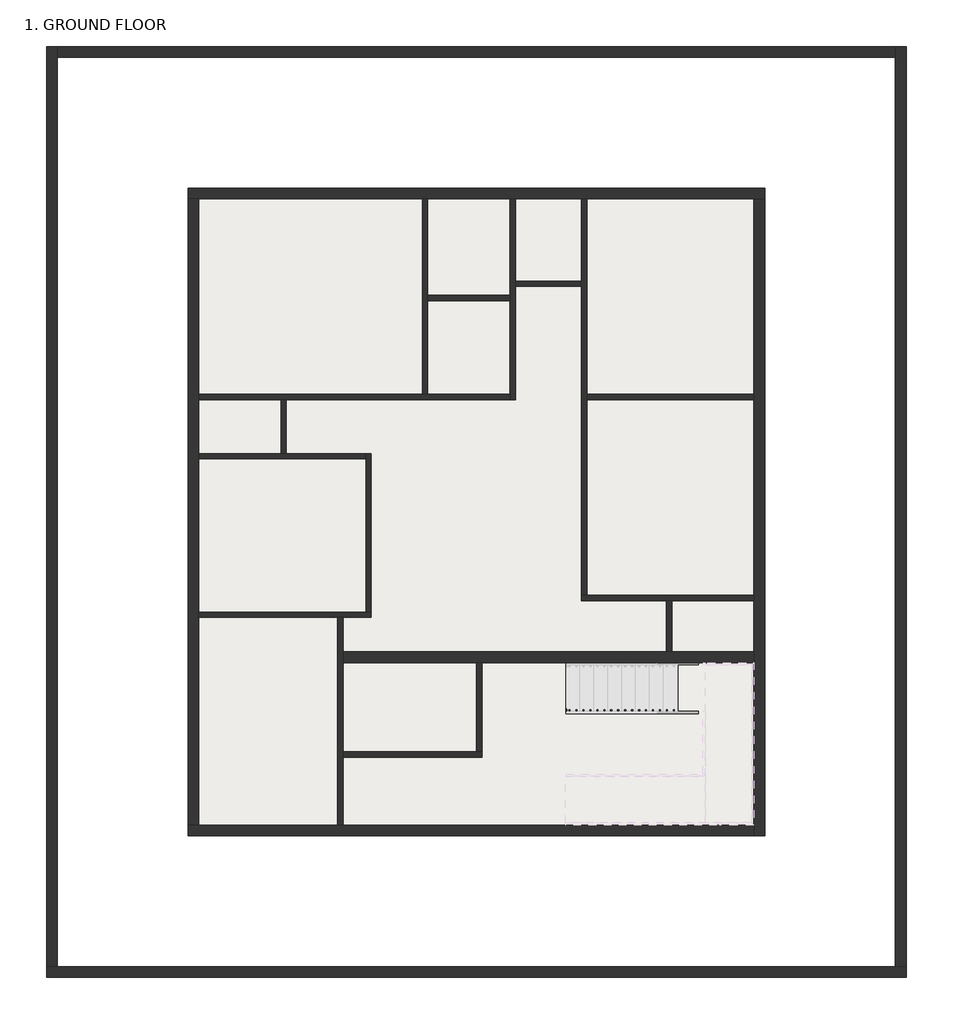
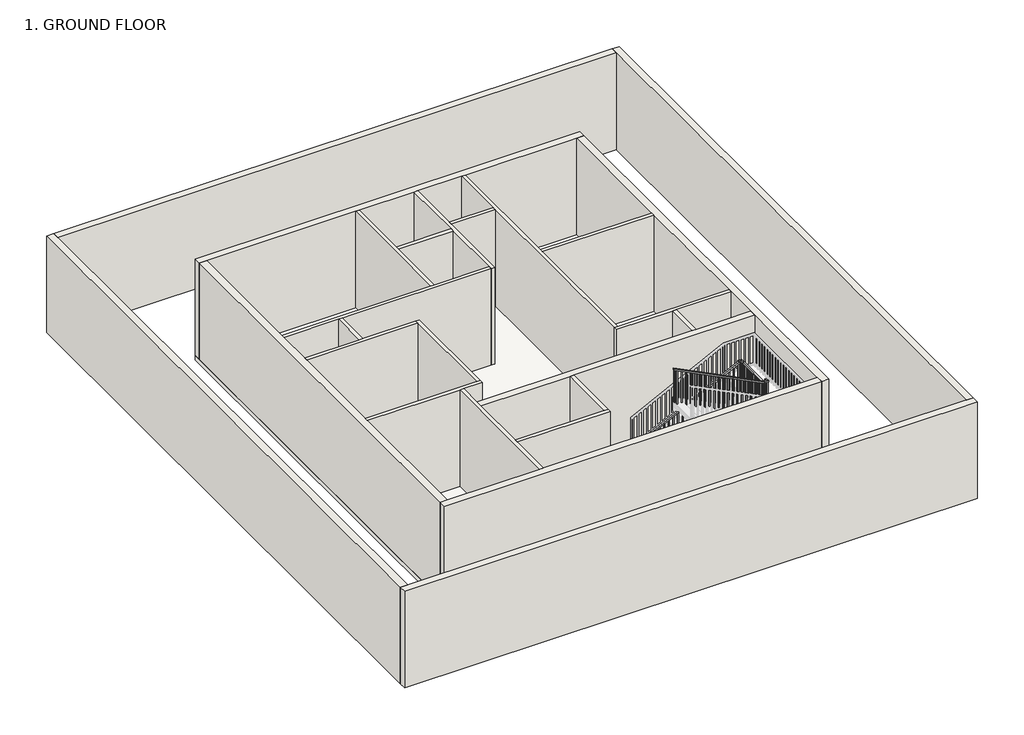
# One storey, part 1 of 2: 25 walls, 3 slabs, 1 railing.
"""IFC4 building model written with IfcOpenShell, lengths in millimetres."""

from ifc_helpers import new_model, si_unit, frame, origin, origin_with_axes, place, context, project, spatial, polyline, outline, extrude, faceted_brep, element, save

model = new_model("IFC4")

# Units and contexts
model_context = context("Model", 3, world=origin())
ifc_project = project(units=[si_unit("LENGTHUNIT", "METRE", prefix="MILLI")], contexts=[model_context])

# Site, building, storey
site = spatial("IfcSite", under=ifc_project)
building = spatial("IfcBuilding", under=site)
storey = spatial("IfcBuildingStorey", under=building, Name="1. GROUND FLOOR", Elevation=0.0)

# Railing
placement = place(None, origin())
element("IfcRailing", 1, ObjectType="1100mm", at=placement, inside=storey, context=model_context, shape_type="SolidModel", body=[
    faceted_brep([(1688.8435815, -3923.691395, 1250.0), (1688.8435815, -3923.691395, 1194.0983006), (1688.8435815, -3973.691395, 1194.0983006), (1688.8435815, -3973.691395, 1250.0), (4614.2435815, -3923.691395, 2712.7), (4664.2435815, -3923.691395, 2681.7983006), (4664.2435815, -3973.691395, 2681.7983006), (4614.2435815, -3973.691395, 2712.7), (4614.2435815, -3923.691395, 2750.0), (4664.2435815, -3923.691395, 2700.0), (4664.2435815, -3973.691395, 2700.0), (4614.2435815, -3973.691395, 2750.0), (4739.2435815, -3923.691395, 2750.0), (4739.2435815, -3923.691395, 2700.0), (4689.2435815, -3973.691395, 2700.0), (4689.2435815, -3973.691395, 2750.0), (4739.2435815, -4048.691395, 2750.0), (4739.2435815, -4048.691395, 2700.0), (4689.2435815, -4048.691395, 2700.0), (4689.2435815, -4048.691395, 2750.0), (4739.2435815, -5301.891395, 2750.0), (4739.2435815, -5351.891395, 2700.0), (4689.2435815, -5351.891395, 2700.0), (4689.2435815, -5301.891395, 2750.0), (4739.2435815, -5301.891395, 2937.3), (4739.2435815, -5351.891395, 2887.3), (4689.2435815, -5351.891395, 2887.3), (4689.2435815, -5301.891395, 2937.3), (4739.2435815, -5426.891395, 2937.3), (4739.2435815, -5426.891395, 2887.3), (4689.2435815, -5376.891395, 2887.3), (4689.2435815, -5376.891395, 2937.3), (4614.2435815, -5426.891395, 2937.3), (4602.4401826, -5426.891395, 2887.3), (4602.4401826, -5376.891395, 2887.3), (4614.2435815, -5376.891395, 2937.3), (1688.8435815, -5426.891395, 4400.0), (1688.8435815, -5376.891395, 4400.0), (1688.8435815, -5376.891395, 4344.0983006), (1688.8435815, -5426.891395, 4344.0983006)], [[[0, 1, 2, 3]], [[1, 0, 4, 5]], [[2, 1, 5, 6]], [[3, 2, 6, 7]], [[0, 3, 7, 4]], [[5, 4, 8, 9]], [[6, 5, 9, 10]], [[7, 6, 10, 11]], [[4, 7, 11, 8]], [[9, 8, 12, 13]], [[10, 9, 13, 14]], [[11, 10, 14, 15]], [[8, 11, 15, 12]], [[13, 12, 16, 17]], [[14, 13, 17, 18]], [[15, 14, 18, 19]], [[12, 15, 19, 16]], [[17, 16, 20, 21]], [[18, 17, 21, 22]], [[19, 18, 22, 23]], [[16, 19, 23, 20]], [[21, 20, 24, 25]], [[22, 21, 25, 26]], [[23, 22, 26, 27]], [[20, 23, 27, 24]], [[25, 24, 28, 29]], [[26, 25, 29, 30]], [[27, 26, 30, 31]], [[24, 27, 31, 28]], [[29, 28, 32, 33]], [[30, 29, 33, 34]], [[31, 30, 34, 35]], [[28, 31, 35, 32]], [[36, 37, 38, 39]], [[33, 32, 36, 39]], [[34, 33, 39, 38]], [[35, 34, 38, 37]], [[32, 35, 37, 36]]]),
    extrude(outline(polyline([(3150.0, 1801.7435815), (4287.6483006, 1801.7435815), (4300.1483006, 1776.7435815), (3150.0, 1776.7435815), (3150.0, 1801.7435815)])), frame((0.0, -5414.391395, 0.0), z_axis=(0.0, 1.0, 0.0), x_axis=(0.0, 0.0, 1.0)), (0.0, 0.0, 1.0), 25.0),
    extrude(outline(polyline([(3150.0, 1951.7435815), (4212.6483006, 1951.7435815), (4225.1483006, 1926.7435815), (3150.0, 1926.7435815), (3150.0, 1951.7435815)])), frame((0.0, -5414.391395, 0.0), z_axis=(0.0, 1.0, 0.0), x_axis=(0.0, 0.0, 1.0)), (0.0, 0.0, 1.0), 25.0),
    extrude(outline(polyline([(3000.0, 2101.7435815), (4137.6483006, 2101.7435815), (4150.1483006, 2076.7435815), (3000.0, 2076.7435815), (3000.0, 2101.7435815)])), frame((0.0, -5414.391395, 0.0), z_axis=(0.0, 1.0, 0.0), x_axis=(0.0, 0.0, 1.0)), (0.0, 0.0, 1.0), 25.0),
    extrude(outline(polyline([(3000.0, 2251.7435815), (4062.6483006, 2251.7435815), (4075.1483006, 2226.7435815), (3000.0, 2226.7435815), (3000.0, 2251.7435815)])), frame((0.0, -5414.391395, 0.0), z_axis=(0.0, 1.0, 0.0), x_axis=(0.0, 0.0, 1.0)), (0.0, 0.0, 1.0), 25.0),
    extrude(outline(polyline([(2850.0, 2401.7435815), (3987.6483006, 2401.7435815), (4000.1483006, 2376.7435815), (2850.0, 2376.7435815), (2850.0, 2401.7435815)])), frame((0.0, -5414.391395, 0.0), z_axis=(0.0, 1.0, 0.0), x_axis=(0.0, 0.0, 1.0)), (0.0, 0.0, 1.0), 25.0),
    extrude(outline(polyline([(2850.0, 2551.7435815), (3912.6483006, 2551.7435815), (3925.1483006, 2526.7435815), (2850.0, 2526.7435815), (2850.0, 2551.7435815)])), frame((0.0, -5414.391395, 0.0), z_axis=(0.0, 1.0, 0.0), x_axis=(0.0, 0.0, 1.0)), (0.0, 0.0, 1.0), 25.0),
    extrude(outline(polyline([(2700.0, 2701.7435815), (3837.6483006, 2701.7435815), (3850.1483006, 2676.7435815), (2700.0, 2676.7435815), (2700.0, 2701.7435815)])), frame((0.0, -5414.391395, 0.0), z_axis=(0.0, 1.0, 0.0), x_axis=(0.0, 0.0, 1.0)), (0.0, 0.0, 1.0), 25.0),
    extrude(outline(polyline([(2700.0, 2851.7435815), (3762.6483006, 2851.7435815), (3775.1483006, 2826.7435815), (2700.0, 2826.7435815), (2700.0, 2851.7435815)])), frame((0.0, -5414.391395, 0.0), z_axis=(0.0, 1.0, 0.0), x_axis=(0.0, 0.0, 1.0)), (0.0, 0.0, 1.0), 25.0),
    extrude(outline(polyline([(2550.0, 3001.7435815), (3687.6483006, 3001.7435815), (3700.1483006, 2976.7435815), (2550.0, 2976.7435815), (2550.0, 3001.7435815)])), frame((0.0, -5414.391395, 0.0), z_axis=(0.0, 1.0, 0.0), x_axis=(0.0, 0.0, 1.0)), (0.0, 0.0, 1.0), 25.0),
    extrude(outline(polyline([(2550.0, 3151.7435815), (3612.6483006, 3151.7435815), (3625.1483006, 3126.7435815), (2550.0, 3126.7435815), (2550.0, 3151.7435815)])), frame((0.0, -5414.391395, 0.0), z_axis=(0.0, 1.0, 0.0), x_axis=(0.0, 0.0, 1.0)), (0.0, 0.0, 1.0), 25.0),
    extrude(outline(polyline([(2400.0, 3301.7435815), (3537.6483006, 3301.7435815), (3550.1483006, 3276.7435815), (2400.0, 3276.7435815), (2400.0, 3301.7435815)])), frame((0.0, -5414.391395, 0.0), z_axis=(0.0, 1.0, 0.0), x_axis=(0.0, 0.0, 1.0)), (0.0, 0.0, 1.0), 25.0),
    extrude(outline(polyline([(2400.0, 3451.7435815), (3462.6483006, 3451.7435815), (3475.1483006, 3426.7435815), (2400.0, 3426.7435815), (2400.0, 3451.7435815)])), frame((0.0, -5414.391395, 0.0), z_axis=(0.0, 1.0, 0.0), x_axis=(0.0, 0.0, 1.0)), (0.0, 0.0, 1.0), 25.0),
    extrude(outline(polyline([(2250.0, 3601.7435815), (3387.6483006, 3601.7435815), (3400.1483006, 3576.7435815), (2250.0, 3576.7435815), (2250.0, 3601.7435815)])), frame((0.0, -5414.391395, 0.0), z_axis=(0.0, 1.0, 0.0), x_axis=(0.0, 0.0, 1.0)), (0.0, 0.0, 1.0), 25.0),
    extrude(outline(polyline([(2250.0, 3751.7435815), (3312.6483006, 3751.7435815), (3325.1483006, 3726.7435815), (2250.0, 3726.7435815), (2250.0, 3751.7435815)])), frame((0.0, -5414.391395, 0.0), z_axis=(0.0, 1.0, 0.0), x_axis=(0.0, 0.0, 1.0)), (0.0, 0.0, 1.0), 25.0),
    extrude(outline(polyline([(2100.0, 3901.7435815), (3237.6483006, 3901.7435815), (3250.1483006, 3876.7435815), (2100.0, 3876.7435815), (2100.0, 3901.7435815)])), frame((0.0, -5414.391395, 0.0), z_axis=(0.0, 1.0, 0.0), x_axis=(0.0, 0.0, 1.0)), (0.0, 0.0, 1.0), 25.0),
    extrude(outline(polyline([(2100.0, 4051.7435815), (3162.6483006, 4051.7435815), (3175.1483006, 4026.7435815), (2100.0, 4026.7435815), (2100.0, 4051.7435815)])), frame((0.0, -5414.391395, 0.0), z_axis=(0.0, 1.0, 0.0), x_axis=(0.0, 0.0, 1.0)), (0.0, 0.0, 1.0), 25.0),
    extrude(outline(polyline([(1950.0, 4201.7435815), (3087.6483006, 4201.7435815), (3100.1483006, 4176.7435815), (1950.0, 4176.7435815), (1950.0, 4201.7435815)])), frame((0.0, -5414.391395, 0.0), z_axis=(0.0, 1.0, 0.0), x_axis=(0.0, 0.0, 1.0)), (0.0, 0.0, 1.0), 25.0),
    extrude(outline(polyline([(1950.0, 4351.7435815), (3012.6483006, 4351.7435815), (3025.1483006, 4326.7435815), (1950.0, 4326.7435815), (1950.0, 4351.7435815)])), frame((0.0, -5414.391395, 0.0), z_axis=(0.0, 1.0, 0.0), x_axis=(0.0, 0.0, 1.0)), (0.0, 0.0, 1.0), 25.0),
    extrude(outline(polyline([(1800.0, 4501.7435815), (2937.6483006, 4501.7435815), (2950.1483006, 4476.7435815), (1800.0, 4476.7435815), (1800.0, 4501.7435815)])), frame((0.0, -5414.391395, 0.0), z_axis=(0.0, 1.0, 0.0), x_axis=(0.0, 0.0, 1.0)), (0.0, 0.0, 1.0), 25.0),
    extrude(outline(polyline([(4651.7435815, -5389.391395), (4651.7435815, -5414.391395), (4626.7435815, -5414.391395), (4626.7435815, -5389.391395), (4651.7435815, -5389.391395)])), frame((0.0, 0.0, 1800.0), z_axis=(0.0, 0.0, 1.0), x_axis=(1.0, 0.0, 0.0)), (0.0, 0.0, 1.0), 1087.3),
    extrude(outline(polyline([(4701.7435815, -5361.191395), (4726.7435815, -5361.191395), (4726.7435815, -5386.191395), (4701.7435815, -5386.191395), (4701.7435815, -5361.191395)])), frame((0.0, 0.0, 1650.0), z_axis=(0.0, 0.0, 1.0), x_axis=(1.0, 0.0, 0.0)), (0.0, 0.0, 1.0), 1237.3),
    extrude(outline(polyline([(4701.7435815, -5211.191395), (4726.7435815, -5211.191395), (4726.7435815, -5236.191395), (4701.7435815, -5236.191395), (4701.7435815, -5211.191395)])), frame((0.0, 0.0, 1650.0), z_axis=(0.0, 0.0, 1.0), x_axis=(1.0, 0.0, 0.0)), (0.0, 0.0, 1.0), 1050.0),
    extrude(outline(polyline([(4701.7435815, -5061.191395), (4726.7435815, -5061.191395), (4726.7435815, -5086.191395), (4701.7435815, -5086.191395), (4701.7435815, -5061.191395)])), frame((0.0, 0.0, 1650.0), z_axis=(0.0, 0.0, 1.0), x_axis=(1.0, 0.0, 0.0)), (0.0, 0.0, 1.0), 1050.0),
    extrude(outline(polyline([(4701.7435815, -4911.191395), (4726.7435815, -4911.191395), (4726.7435815, -4936.191395), (4701.7435815, -4936.191395), (4701.7435815, -4911.191395)])), frame((0.0, 0.0, 1650.0), z_axis=(0.0, 0.0, 1.0), x_axis=(1.0, 0.0, 0.0)), (0.0, 0.0, 1.0), 1050.0),
    extrude(outline(polyline([(4701.7435815, -4761.191395), (4726.7435815, -4761.191395), (4726.7435815, -4786.191395), (4701.7435815, -4786.191395), (4701.7435815, -4761.191395)])), frame((0.0, 0.0, 1650.0), z_axis=(0.0, 0.0, 1.0), x_axis=(1.0, 0.0, 0.0)), (0.0, 0.0, 1.0), 1050.0),
    extrude(outline(polyline([(4701.7435815, -4611.191395), (4726.7435815, -4611.191395), (4726.7435815, -4636.191395), (4701.7435815, -4636.191395), (4701.7435815, -4611.191395)])), frame((0.0, 0.0, 1650.0), z_axis=(0.0, 0.0, 1.0), x_axis=(1.0, 0.0, 0.0)), (0.0, 0.0, 1.0), 1050.0),
    extrude(outline(polyline([(4701.7435815, -4461.191395), (4726.7435815, -4461.191395), (4726.7435815, -4486.191395), (4701.7435815, -4486.191395), (4701.7435815, -4461.191395)])), frame((0.0, 0.0, 1650.0), z_axis=(0.0, 0.0, 1.0), x_axis=(1.0, 0.0, 0.0)), (0.0, 0.0, 1.0), 1050.0),
    extrude(outline(polyline([(4701.7435815, -4311.191395), (4726.7435815, -4311.191395), (4726.7435815, -4336.191395), (4701.7435815, -4336.191395), (4701.7435815, -4311.191395)])), frame((0.0, 0.0, 1650.0), z_axis=(0.0, 0.0, 1.0), x_axis=(1.0, 0.0, 0.0)), (0.0, 0.0, 1.0), 1050.0),
    extrude(outline(polyline([(4701.7435815, -4161.191395), (4726.7435815, -4161.191395), (4726.7435815, -4186.191395), (4701.7435815, -4186.191395), (4701.7435815, -4161.191395)])), frame((0.0, 0.0, 1650.0), z_axis=(0.0, 0.0, 1.0), x_axis=(1.0, 0.0, 0.0)), (0.0, 0.0, 1.0), 1050.0),
    extrude(outline(polyline([(4701.7435815, -4011.191395), (4726.7435815, -4011.191395), (4726.7435815, -4036.191395), (4701.7435815, -4036.191395), (4701.7435815, -4011.191395)])), frame((0.0, 0.0, 1650.0), z_axis=(0.0, 0.0, 1.0), x_axis=(1.0, 0.0, 0.0)), (0.0, 0.0, 1.0), 1050.0),
    extrude(outline(polyline([(2650.3483006, 4601.3435815), (1500.0, 4601.3435815), (1500.0, 4626.3435815), (2662.8483006, 4626.3435815), (2650.3483006, 4601.3435815)])), frame((0.0, -3961.191395, 0.0), z_axis=(0.0, 1.0, 0.0), x_axis=(0.0, 0.0, 1.0)), (0.0, 0.0, 1.0), 25.0),
    extrude(outline(polyline([(2575.3483006, 4451.3435815), (1500.0, 4451.3435815), (1500.0, 4476.3435815), (2587.8483006, 4476.3435815), (2575.3483006, 4451.3435815)])), frame((0.0, -3961.191395, 0.0), z_axis=(0.0, 1.0, 0.0), x_axis=(0.0, 0.0, 1.0)), (0.0, 0.0, 1.0), 25.0),
    extrude(outline(polyline([(2500.3483006, 4301.3435815), (1350.0, 4301.3435815), (1350.0, 4326.3435815), (2512.8483006, 4326.3435815), (2500.3483006, 4301.3435815)])), frame((0.0, -3961.191395, 0.0), z_axis=(0.0, 1.0, 0.0), x_axis=(0.0, 0.0, 1.0)), (0.0, 0.0, 1.0), 25.0),
    extrude(outline(polyline([(2425.3483006, 4151.3435815), (1350.0, 4151.3435815), (1350.0, 4176.3435815), (2437.8483006, 4176.3435815), (2425.3483006, 4151.3435815)])), frame((0.0, -3961.191395, 0.0), z_axis=(0.0, 1.0, 0.0), x_axis=(0.0, 0.0, 1.0)), (0.0, 0.0, 1.0), 25.0),
    extrude(outline(polyline([(2350.3483006, 4001.3435815), (1200.0, 4001.3435815), (1200.0, 4026.3435815), (2362.8483006, 4026.3435815), (2350.3483006, 4001.3435815)])), frame((0.0, -3961.191395, 0.0), z_axis=(0.0, 1.0, 0.0), x_axis=(0.0, 0.0, 1.0)), (0.0, 0.0, 1.0), 25.0),
    extrude(outline(polyline([(2275.3483006, 3851.3435815), (1200.0, 3851.3435815), (1200.0, 3876.3435815), (2287.8483006, 3876.3435815), (2275.3483006, 3851.3435815)])), frame((0.0, -3961.191395, 0.0), z_axis=(0.0, 1.0, 0.0), x_axis=(0.0, 0.0, 1.0)), (0.0, 0.0, 1.0), 25.0),
    extrude(outline(polyline([(2200.3483006, 3701.3435815), (1050.0, 3701.3435815), (1050.0, 3726.3435815), (2212.8483006, 3726.3435815), (2200.3483006, 3701.3435815)])), frame((0.0, -3961.191395, 0.0), z_axis=(0.0, 1.0, 0.0), x_axis=(0.0, 0.0, 1.0)), (0.0, 0.0, 1.0), 25.0),
    extrude(outline(polyline([(2125.3483006, 3551.3435815), (1050.0, 3551.3435815), (1050.0, 3576.3435815), (2137.8483006, 3576.3435815), (2125.3483006, 3551.3435815)])), frame((0.0, -3961.191395, 0.0), z_axis=(0.0, 1.0, 0.0), x_axis=(0.0, 0.0, 1.0)), (0.0, 0.0, 1.0), 25.0),
    extrude(outline(polyline([(2050.3483006, 3401.3435815), (900.0, 3401.3435815), (900.0, 3426.3435815), (2062.8483006, 3426.3435815), (2050.3483006, 3401.3435815)])), frame((0.0, -3961.191395, 0.0), z_axis=(0.0, 1.0, 0.0), x_axis=(0.0, 0.0, 1.0)), (0.0, 0.0, 1.0), 25.0),
    extrude(outline(polyline([(1975.3483006, 3251.3435815), (900.0, 3251.3435815), (900.0, 3276.3435815), (1987.8483006, 3276.3435815), (1975.3483006, 3251.3435815)])), frame((0.0, -3961.191395, 0.0), z_axis=(0.0, 1.0, 0.0), x_axis=(0.0, 0.0, 1.0)), (0.0, 0.0, 1.0), 25.0),
    extrude(outline(polyline([(1900.3483006, 3101.3435815), (750.0, 3101.3435815), (750.0, 3126.3435815), (1912.8483006, 3126.3435815), (1900.3483006, 3101.3435815)])), frame((0.0, -3961.191395, 0.0), z_axis=(0.0, 1.0, 0.0), x_axis=(0.0, 0.0, 1.0)), (0.0, 0.0, 1.0), 25.0),
    extrude(outline(polyline([(1825.3483006, 2951.3435815), (750.0, 2951.3435815), (750.0, 2976.3435815), (1837.8483006, 2976.3435815), (1825.3483006, 2951.3435815)])), frame((0.0, -3961.191395, 0.0), z_axis=(0.0, 1.0, 0.0), x_axis=(0.0, 0.0, 1.0)), (0.0, 0.0, 1.0), 25.0),
    extrude(outline(polyline([(1750.3483006, 2801.3435815), (600.0, 2801.3435815), (600.0, 2826.3435815), (1762.8483006, 2826.3435815), (1750.3483006, 2801.3435815)])), frame((0.0, -3961.191395, 0.0), z_axis=(0.0, 1.0, 0.0), x_axis=(0.0, 0.0, 1.0)), (0.0, 0.0, 1.0), 25.0),
    extrude(outline(polyline([(1675.3483006, 2651.3435815), (600.0, 2651.3435815), (600.0, 2676.3435815), (1687.8483006, 2676.3435815), (1675.3483006, 2651.3435815)])), frame((0.0, -3961.191395, 0.0), z_axis=(0.0, 1.0, 0.0), x_axis=(0.0, 0.0, 1.0)), (0.0, 0.0, 1.0), 25.0),
    extrude(outline(polyline([(1600.3483006, 2501.3435815), (450.0, 2501.3435815), (450.0, 2526.3435815), (1612.8483006, 2526.3435815), (1600.3483006, 2501.3435815)])), frame((0.0, -3961.191395, 0.0), z_axis=(0.0, 1.0, 0.0), x_axis=(0.0, 0.0, 1.0)), (0.0, 0.0, 1.0), 25.0),
    extrude(outline(polyline([(1525.3483006, 2351.3435815), (450.0, 2351.3435815), (450.0, 2376.3435815), (1537.8483006, 2376.3435815), (1525.3483006, 2351.3435815)])), frame((0.0, -3961.191395, 0.0), z_axis=(0.0, 1.0, 0.0), x_axis=(0.0, 0.0, 1.0)), (0.0, 0.0, 1.0), 25.0),
    extrude(outline(polyline([(1450.3483006, 2201.3435815), (300.0, 2201.3435815), (300.0, 2226.3435815), (1462.8483006, 2226.3435815), (1450.3483006, 2201.3435815)])), frame((0.0, -3961.191395, 0.0), z_axis=(0.0, 1.0, 0.0), x_axis=(0.0, 0.0, 1.0)), (0.0, 0.0, 1.0), 25.0),
    extrude(outline(polyline([(1375.3483006, 2051.3435815), (300.0, 2051.3435815), (300.0, 2076.3435815), (1387.8483006, 2076.3435815), (1375.3483006, 2051.3435815)])), frame((0.0, -3961.191395, 0.0), z_axis=(0.0, 1.0, 0.0), x_axis=(0.0, 0.0, 1.0)), (0.0, 0.0, 1.0), 25.0),
    extrude(outline(polyline([(1300.3483006, 1901.3435815), (150.0, 1901.3435815), (150.0, 1926.3435815), (1312.8483006, 1926.3435815), (1300.3483006, 1901.3435815)])), frame((0.0, -3961.191395, 0.0), z_axis=(0.0, 1.0, 0.0), x_axis=(0.0, 0.0, 1.0)), (0.0, 0.0, 1.0), 25.0),
    extrude(outline(polyline([(1225.3483006, 1751.3435815), (150.0, 1751.3435815), (150.0, 1776.3435815), (1237.8483006, 1776.3435815), (1225.3483006, 1751.3435815)])), frame((0.0, -3961.191395, 0.0), z_axis=(0.0, 1.0, 0.0), x_axis=(0.0, 0.0, 1.0)), (0.0, 0.0, 1.0), 25.0),
    extrude(outline(polyline([(4701.7435815, -5389.391395), (4726.7435815, -5389.391395), (4726.7435815, -5414.391395), (4701.7435815, -5414.391395), (4701.7435815, -5389.391395)])), frame((0.0, 0.0, 1650.0), z_axis=(0.0, 0.0, 1.0), x_axis=(1.0, 0.0, 0.0)), (0.0, 0.0, 1.0), 1237.3),
    extrude(outline(polyline([(4701.7435815, -3961.191395), (4701.7435815, -3936.191395), (4726.7435815, -3936.191395), (4726.7435815, -3961.191395), (4701.7435815, -3961.191395)])), frame((0.0, 0.0, 1650.0), z_axis=(0.0, 0.0, 1.0), x_axis=(1.0, 0.0, 0.0)), (0.0, 0.0, 1.0), 1050.0),
    extrude(outline(polyline([(3150.0, 1713.8435815), (4331.5983006, 1713.8435815), (4344.0983006, 1688.8435815), (3150.0, 1688.8435815), (3150.0, 1713.8435815)])), frame((0.0, -5414.391395, 0.0), z_axis=(0.0, 1.0, 0.0), x_axis=(0.0, 0.0, 1.0)), (0.0, 0.0, 1.0), 25.0),
    extrude(outline(polyline([(1194.0983006, 1688.8435815), (150.0, 1688.8435815), (150.0, 1713.8435815), (1206.5983006, 1713.8435815), (1194.0983006, 1688.8435815)])), frame((0.0, -3961.191395, 0.0), z_axis=(0.0, 1.0, 0.0), x_axis=(0.0, 0.0, 1.0)), (0.0, 0.0, 1.0), 25.0),
])

# Slabs
element("IfcSlab", 2, at=placement, inside=storey, context=model_context, shape_type="SweptSolid", body=[
    extrude(outline(polyline([(482.4435815, 7059.508605), (482.4435815, 4983.408605), (-1288.8564185, 4983.408605), (-1288.8564185, 7059.508605), (482.4435815, 7059.508605)])), frame((0.0, 0.0, -200.0), z_axis=(0.0, 0.0, 1.0), x_axis=(1.0, 0.0, 0.0)), (0.0, 0.0, 1.0), 200.0),
    extrude(outline(polyline([(5738.8435815, -1589.891395), (5738.8435815, -2694.091395), (3967.5435815, -2694.091395), (3967.5435815, -1589.891395), (5738.8435815, -1589.891395)])), frame((0.0, 0.0, -200.0), z_axis=(0.0, 0.0, 1.0), x_axis=(1.0, 0.0, 0.0)), (0.0, 0.0, 1.0), 200.0),
    extrude(outline(polyline([(-4451.8564185, 2734.808605), (-4451.8564185, 1573.108605), (-6223.1564185, 1573.108605), (-6223.1564185, 2734.808605), (-4451.8564185, 2734.808605)])), frame((0.0, 0.0, -200.0), z_axis=(0.0, 0.0, 1.0), x_axis=(1.0, 0.0, 0.0)), (0.0, 0.0, 1.0), 200.0),
])
element("IfcSlab", 3, ObjectType="Generic 150mm", at=placement, inside=storey, context=model_context, shape_type="SweptSolid", body=[
    extrude(outline(polyline([(5968.8435815, 7289.508605), (5968.8435815, -6656.491395), (-6453.1564185, -6656.491395), (-6453.1564185, 7289.508605), (5968.8435815, 7289.508605)]), holes=[polyline([(5738.8435815, -1589.891395), (3967.5435815, -1589.891395), (3967.5435815, -2694.091395), (5738.8435815, -2694.091395), (5738.8435815, -1589.891395)]), polyline([(-4451.8564185, 2734.808605), (-6223.1564185, 2734.808605), (-6223.1564185, 1573.108605), (-4451.8564185, 1573.108605), (-4451.8564185, 2734.808605)]), polyline([(-1288.8564185, 4983.408605), (482.4435815, 4983.408605), (482.4435815, 7059.508605), (-1288.8564185, 7059.508605), (-1288.8564185, 4983.408605)])]), frame((0.0, 0.0, -150.0), z_axis=(0.0, 0.0, 1.0), x_axis=(1.0, 0.0, 0.0)), (0.0, 0.0, 1.0), 150.0),
])
element("IfcSlab", 4, ObjectType="Generic 150mm", at=placement, inside=storey, context=model_context, shape_type="SweptSolid", body=[
    extrude(outline(polyline([(-1288.8564185, 4983.408605), (-1288.8564185, 7059.508605), (482.4435815, 7059.508605), (482.4435815, 4983.408605), (-1288.8564185, 4983.408605)])), frame((0.0, 0.0, -350.0), z_axis=(0.0, 0.0, 1.0), x_axis=(1.0, 0.0, 0.0)), (0.0, 0.0, 1.0), 150.0),
    extrude(outline(polyline([(5738.8435815, -2694.091395), (3967.5435815, -2694.091395), (3967.5435815, -1589.891395), (5738.8435815, -1589.891395), (5738.8435815, -2694.091395)])), frame((0.0, 0.0, -350.0), z_axis=(0.0, 0.0, 1.0), x_axis=(1.0, 0.0, 0.0)), (0.0, 0.0, 1.0), 150.0),
    extrude(outline(polyline([(-4451.8564185, 2734.808605), (-4451.8564185, 1573.108605), (-6223.1564185, 1573.108605), (-6223.1564185, 2734.808605), (-4451.8564185, 2734.808605)])), frame((0.0, 0.0, -350.0), z_axis=(0.0, 0.0, 1.0), x_axis=(1.0, 0.0, 0.0)), (0.0, 0.0, 1.0), 150.0),
])

# Walls
element("IfcWall", 5, ObjectType="Generic - 115 mm", at=placement, inside=storey, context=model_context, shape_type="Brep", body=[
    faceted_brep([(-1403.8564185, 7059.508605, 0.0), (-1403.8564185, 2849.808605, 0.0), (-1403.8564185, 2849.808605, 3300.0), (-1403.8564185, 7059.508605, 3300.0), (-1288.8564185, 7059.508605, 0.0), (-1288.8564185, 7059.508605, 3300.0), (-1288.8564185, 4983.408605, 3300.0), (-1288.8564185, 4868.408605, 3300.0), (-1288.8564185, 2849.808605, 3300.0), (-1288.8564185, 2849.808605, 0.0), (-1288.8564185, 4868.408605, 0.0), (-1288.8564185, 4983.408605, 0.0)], [[[0, 1, 2, 3]], [[4, 5, 6, 7, 8, 9, 10, 11]], [[1, 0, 4, 11, 10, 9]], [[3, 2, 8, 7, 6, 5]], [[0, 3, 5, 4]], [[2, 1, 9, 8]]]),
])
element("IfcWall", 6, ObjectType="Generic - 115 mm", at=placement, inside=storey, context=model_context, shape_type="Brep", body=[
    faceted_brep([(482.4435815, 2849.808605, 0.0), (-1288.8564185, 2849.808605, 0.0), (-1403.8564185, 2849.808605, 0.0), (-6223.1564185, 2849.808605, 0.0), (-6223.1564185, 2849.808605, 3300.0), (-1403.8564185, 2849.808605, 3300.0), (-1288.8564185, 2849.808605, 3300.0), (482.4435815, 2849.808605, 3300.0), (482.4435815, 2734.808605, 0.0), (482.4435815, 2734.808605, 3300.0), (-4336.8564185, 2734.808605, 3300.0), (-4451.8564185, 2734.808605, 3300.0), (-6223.1564185, 2734.808605, 3300.0), (-6223.1564185, 2734.808605, 0.0), (-4451.8564185, 2734.808605, 0.0), (-4336.8564185, 2734.808605, 0.0)], [[[0, 1, 2, 3, 4, 5, 6, 7]], [[8, 9, 10, 11, 12, 13, 14, 15]], [[3, 2, 1, 0, 8, 15, 14, 13]], [[7, 6, 5, 4, 12, 11, 10, 9]], [[4, 3, 13, 12]], [[0, 7, 9, 8]]]),
])
element("IfcWall", 7, ObjectType="Generic - 115 mm", at=placement, inside=storey, context=model_context, shape_type="Brep", body=[
    faceted_brep([(482.4435815, 7059.508605, 0.0), (482.4435815, 4983.408605, 0.0), (482.4435815, 4868.408605, 0.0), (482.4435815, 2849.808605, 0.0), (482.4435815, 2734.808605, 0.0), (482.4435815, 2734.808605, 3300.0), (482.4435815, 2849.808605, 3300.0), (482.4435815, 4868.408605, 3300.0), (482.4435815, 4983.408605, 3300.0), (482.4435815, 7059.508605, 3300.0), (597.4435815, 7059.508605, 0.0), (597.4435815, 7059.508605, 3300.0), (597.4435815, 5288.208605, 3300.0), (597.4435815, 5173.208605, 3300.0), (597.4435815, 2734.808605, 3300.0), (597.4435815, 2734.808605, 0.0), (597.4435815, 5173.208605, 0.0), (597.4435815, 5288.208605, 0.0)], [[[0, 1, 2, 3, 4, 5, 6, 7, 8, 9]], [[10, 11, 12, 13, 14, 15, 16, 17]], [[4, 3, 2, 1, 0, 10, 17, 16, 15]], [[9, 8, 7, 6, 5, 14, 13, 12, 11]], [[0, 9, 11, 10]], [[5, 4, 15, 14]]]),
])
element("IfcWall", 8, ObjectType="Generic - 115 mm", at=placement, inside=storey, context=model_context, shape_type="SweptSolid", body=[
    extrude(outline(polyline([(482.4435815, 4868.408605), (-1288.8564185, 4868.408605), (-1288.8564185, 4983.408605), (482.4435815, 4983.408605), (482.4435815, 4868.408605)])), origin_with_axes(), (0.0, 0.0, 1.0), 3300.0),
])
element("IfcWall", 9, ObjectType="Generic - 115 mm", at=placement, inside=storey, context=model_context, shape_type="Brep", body=[
    faceted_brep([(2023.7435815, 7059.508605, 0.0), (2023.7435815, 5288.208605, 0.0), (2023.7435815, 5173.208605, 0.0), (2023.7435815, -1474.891395, 0.0), (2023.7435815, -1474.891395, 3300.0), (2023.7435815, 5173.208605, 3300.0), (2023.7435815, 5288.208605, 3300.0), (2023.7435815, 7059.508605, 3300.0), (2138.7435815, 7059.508605, 0.0), (2138.7435815, 7059.508605, 3300.0), (2138.7435815, 2849.808605, 3300.0), (2138.7435815, 2734.808605, 3300.0), (2138.7435815, -1474.891395, 3300.0), (2138.7435815, -1474.891395, 0.0), (2138.7435815, 2734.808605, 0.0), (2138.7435815, 2849.808605, 0.0)], [[[0, 1, 2, 3, 4, 5, 6, 7]], [[8, 9, 10, 11, 12, 13, 14, 15]], [[3, 2, 1, 0, 8, 15, 14, 13]], [[7, 6, 5, 4, 12, 11, 10, 9]], [[0, 7, 9, 8]], [[4, 3, 13, 12]]]),
])
element("IfcWall", 10, ObjectType="Generic - 115 mm", at=placement, inside=storey, context=model_context, shape_type="SweptSolid", body=[
    extrude(outline(polyline([(5738.8435815, 2734.808605), (2138.7435815, 2734.808605), (2138.7435815, 2849.808605), (5738.8435815, 2849.808605), (5738.8435815, 2734.808605)])), origin_with_axes(), (0.0, 0.0, 1.0), 3300.0),
])
element("IfcWall", 11, ObjectType="Generic - 115 mm", at=placement, inside=storey, context=model_context, shape_type="SweptSolid", body=[
    extrude(outline(polyline([(2023.7435815, 5173.208605), (597.4435815, 5173.208605), (597.4435815, 5288.208605), (2023.7435815, 5288.208605), (2023.7435815, 5173.208605)])), origin_with_axes(), (0.0, 0.0, 1.0), 3300.0),
])
element("IfcWall", 12, ObjectType="Generic - 115 mm", at=placement, inside=storey, context=model_context, shape_type="Brep", body=[
    faceted_brep([(5738.8435815, -1474.891395, 0.0), (2138.7435815, -1474.891395, 0.0), (2023.7435815, -1474.891395, 0.0), (2023.7435815, -1474.891395, 3300.0), (2138.7435815, -1474.891395, 3300.0), (5738.8435815, -1474.891395, 3300.0), (5738.8435815, -1589.891395, 0.0), (5738.8435815, -1589.891395, 3300.0), (3967.5435815, -1589.891395, 3300.0), (3852.5435815, -1589.891395, 3300.0), (2023.7435815, -1589.891395, 3300.0), (2023.7435815, -1589.891395, 0.0), (3852.5435815, -1589.891395, 0.0), (3967.5435815, -1589.891395, 0.0)], [[[0, 1, 2, 3, 4, 5]], [[6, 7, 8, 9, 10, 11, 12, 13]], [[2, 1, 0, 6, 13, 12, 11]], [[5, 4, 3, 10, 9, 8, 7]], [[0, 5, 7, 6]], [[3, 2, 11, 10]]]),
])
element("IfcWall", 13, ObjectType="Generic - 115 mm", at=placement, inside=storey, context=model_context, shape_type="SweptSolid", body=[
    extrude(outline(polyline([(3967.5435815, -1589.891395), (3967.5435815, -2694.091395), (3852.5435815, -2694.091395), (3852.5435815, -1589.891395), (3967.5435815, -1589.891395)])), origin_with_axes(), (0.0, 0.0, 1.0), 3300.0),
])
element("IfcWall", 14, ObjectType="Generic - 115 mm", at=placement, inside=storey, context=model_context, shape_type="Brep", body=[
    faceted_brep([(-6223.1564185, 1458.108605, 0.0), (-2623.0564185, 1458.108605, 0.0), (-2623.0564185, 1458.108605, 3300.0), (-6223.1564185, 1458.108605, 3300.0), (-6223.1564185, 1573.108605, 0.0), (-6223.1564185, 1573.108605, 3300.0), (-4451.8564185, 1573.108605, 3300.0), (-4336.8564185, 1573.108605, 3300.0), (-2623.0564185, 1573.108605, 3300.0), (-2623.0564185, 1573.108605, 0.0), (-4336.8564185, 1573.108605, 0.0), (-4451.8564185, 1573.108605, 0.0)], [[[0, 1, 2, 3]], [[4, 5, 6, 7, 8, 9, 10, 11]], [[1, 0, 4, 11, 10, 9]], [[3, 2, 8, 7, 6, 5]], [[0, 3, 5, 4]], [[2, 1, 9, 8]]]),
])
element("IfcWall", 15, ObjectType="Generic - 115 mm", at=placement, inside=storey, context=model_context, shape_type="SweptSolid", body=[
    extrude(outline(polyline([(-4336.8564185, 2734.808605), (-4336.8564185, 1573.108605), (-4451.8564185, 1573.108605), (-4451.8564185, 2734.808605), (-4336.8564185, 2734.808605)])), origin_with_axes(), (0.0, 0.0, 1.0), 3300.0),
])
element("IfcWall", 16, ObjectType="Generic - 115 mm", at=placement, inside=storey, context=model_context, shape_type="Brep", body=[
    faceted_brep([(-6223.1564185, -1952.191395, 0.0), (-3232.6564185, -1952.191395, 0.0), (-3117.6564185, -1952.191395, 0.0), (-2508.0564185, -1952.191395, 0.0), (-2508.0564185, -1952.191395, 3300.0), (-3117.6564185, -1952.191395, 3300.0), (-3232.6564185, -1952.191395, 3300.0), (-6223.1564185, -1952.191395, 3300.0), (-6223.1564185, -1837.191395, 0.0), (-6223.1564185, -1837.191395, 3300.0), (-2623.0564185, -1837.191395, 3300.0), (-2508.0564185, -1837.191395, 3300.0), (-2508.0564185, -1837.191395, 0.0), (-2623.0564185, -1837.191395, 0.0)], [[[0, 1, 2, 3, 4, 5, 6, 7]], [[8, 9, 10, 11, 12, 13]], [[3, 2, 1, 0, 8, 13, 12]], [[7, 6, 5, 4, 11, 10, 9]], [[0, 7, 9, 8]], [[4, 3, 12, 11]]]),
])
element("IfcWall", 17, ObjectType="Generic - 115 mm", at=placement, inside=storey, context=model_context, shape_type="Brep", body=[
    faceted_brep([(-2508.0564185, -1837.191395, 0.0), (-2508.0564185, 1573.108605, 0.0), (-2508.0564185, 1573.108605, 3300.0), (-2508.0564185, -1837.191395, 3300.0), (-2623.0564185, -1837.191395, 0.0), (-2623.0564185, -1837.191395, 3300.0), (-2623.0564185, 1458.108605, 3300.0), (-2623.0564185, 1573.108605, 3300.0), (-2623.0564185, 1573.108605, 0.0), (-2623.0564185, 1458.108605, 0.0)], [[[0, 1, 2, 3]], [[4, 5, 6, 7, 8, 9]], [[1, 0, 4, 9, 8]], [[3, 2, 7, 6, 5]], [[0, 3, 5, 4]], [[2, 1, 8, 7]]]),
])
element("IfcWall", 18, ObjectType="Generic - 115 mm", at=placement, inside=storey, context=model_context, shape_type="Brep", body=[
    faceted_brep([(-3117.6564185, -6426.491395, 0.0), (-3117.6564185, -4959.991395, 0.0), (-3117.6564185, -4844.991395, 0.0), (-3117.6564185, -2924.091395, 0.0), (-3117.6564185, -2694.091395, 0.0), (-3117.6564185, -1952.191395, 0.0), (-3117.6564185, -1952.191395, 3300.0), (-3117.6564185, -2694.091395, 3300.0), (-3117.6564185, -2924.091395, 3300.0), (-3117.6564185, -4844.991395, 3300.0), (-3117.6564185, -4959.991395, 3300.0), (-3117.6564185, -6426.491395, 3300.0), (-3232.6564185, -6426.491395, 0.0), (-3232.6564185, -6426.491395, 3300.0), (-3232.6564185, -1952.191395, 3300.0), (-3232.6564185, -1952.191395, 0.0)], [[[0, 1, 2, 3, 4, 5, 6, 7, 8, 9, 10, 11]], [[12, 13, 14, 15]], [[5, 4, 3, 2, 1, 0, 12, 15]], [[11, 10, 9, 8, 7, 6, 14, 13]], [[6, 5, 15, 14]], [[0, 11, 13, 12]]]),
])
element("IfcWall", 19, ObjectType="Generic - 115 mm", at=placement, inside=storey, context=model_context, shape_type="Brep", body=[
    faceted_brep([(-3117.6564185, -4959.991395, 0.0), (-118.7564185, -4959.991395, 0.0), (-118.7564185, -4959.991395, 3300.0), (-3117.6564185, -4959.991395, 3300.0), (-3117.6564185, -4844.991395, 0.0), (-3117.6564185, -4844.991395, 3300.0), (-233.7564185, -4844.991395, 3300.0), (-118.7564185, -4844.991395, 3300.0), (-118.7564185, -4844.991395, 0.0), (-233.7564185, -4844.991395, 0.0)], [[[0, 1, 2, 3]], [[4, 5, 6, 7, 8, 9]], [[1, 0, 4, 9, 8]], [[3, 2, 7, 6, 5]], [[0, 3, 5, 4]], [[2, 1, 8, 7]]]),
])
element("IfcWall", 20, ObjectType="Generic - 115 mm", at=placement, inside=storey, context=model_context, shape_type="SweptSolid", body=[
    extrude(outline(polyline([(-233.7564185, -4844.991395), (-233.7564185, -2924.091395), (-118.7564185, -2924.091395), (-118.7564185, -4844.991395), (-233.7564185, -4844.991395)])), origin_with_axes(), (0.0, 0.0, 1.0), 3300.0),
])
element("IfcWall", 21, ObjectType="Generic - 230 mm", at=placement, inside=storey, context=model_context, shape_type="Brep", body=[
    faceted_brep([(-6453.1564185, 7059.508605, 0.0), (-6223.1564185, 7059.508605, 0.0), (-1403.8564185, 7059.508605, 0.0), (-1288.8564185, 7059.508605, 0.0), (482.4435815, 7059.508605, 0.0), (597.4435815, 7059.508605, 0.0), (2023.7435815, 7059.508605, 0.0), (2138.7435815, 7059.508605, 0.0), (5738.8435815, 7059.508605, 0.0), (5968.8435815, 7059.508605, 0.0), (5968.8435815, 7059.508605, 3300.0), (5738.8435815, 7059.508605, 3300.0), (2138.7435815, 7059.508605, 3300.0), (2023.7435815, 7059.508605, 3300.0), (597.4435815, 7059.508605, 3300.0), (482.4435815, 7059.508605, 3300.0), (-1288.8564185, 7059.508605, 3300.0), (-1403.8564185, 7059.508605, 3300.0), (-6223.1564185, 7059.508605, 3300.0), (-6453.1564185, 7059.508605, 3300.0), (-6453.1564185, 7289.508605, 0.0), (-6453.1564185, 7289.508605, 3300.0), (5968.8435815, 7289.508605, 3300.0), (5968.8435815, 7289.508605, 0.0)], [[[0, 1, 2, 3, 4, 5, 6, 7, 8, 9, 10, 11, 12, 13, 14, 15, 16, 17, 18, 19]], [[20, 21, 22, 23]], [[9, 8, 7, 6, 5, 4, 3, 2, 1, 0, 20, 23]], [[19, 18, 17, 16, 15, 14, 13, 12, 11, 10, 22, 21]], [[10, 9, 23, 22]], [[0, 19, 21, 20]]]),
])
element("IfcWall", 22, ObjectType="Generic - 230 mm", at=placement, inside=storey, context=model_context, shape_type="Brep", body=[
    faceted_brep([(5738.8435815, 7059.508605, 0.0), (5738.8435815, 2849.808605, 0.0), (5738.8435815, 2734.808605, 0.0), (5738.8435815, -1474.891395, 0.0), (5738.8435815, -1589.891395, 0.0), (5738.8435815, -2694.091395, 0.0), (5738.8435815, -2924.091395, 0.0), (5738.8435815, -6426.491395, 0.0), (5738.8435815, -6656.491395, 0.0), (5738.8435815, -6656.491395, 3300.0), (5738.8435815, -6426.491395, 3300.0), (5738.8435815, -2924.091395, 3300.0), (5738.8435815, -2694.091395, 3300.0), (5738.8435815, -1589.891395, 3300.0), (5738.8435815, -1474.891395, 3300.0), (5738.8435815, 2734.808605, 3300.0), (5738.8435815, 2849.808605, 3300.0), (5738.8435815, 7059.508605, 3300.0), (5968.8435815, 7059.508605, 0.0), (5968.8435815, 7059.508605, 3300.0), (5968.8435815, -6656.491395, 3300.0), (5968.8435815, -6656.491395, 0.0)], [[[0, 1, 2, 3, 4, 5, 6, 7, 8, 9, 10, 11, 12, 13, 14, 15, 16, 17]], [[18, 19, 20, 21]], [[8, 7, 6, 5, 4, 3, 2, 1, 0, 18, 21]], [[17, 16, 15, 14, 13, 12, 11, 10, 9, 20, 19]], [[0, 17, 19, 18]], [[9, 8, 21, 20]]]),
])
element("IfcWall", 23, ObjectType="Generic - 230 mm", at=placement, inside=storey, context=model_context, shape_type="Brep", body=[
    faceted_brep([(5738.8435815, -6426.491395, 0.0), (-3117.6564185, -6426.491395, 0.0), (-3232.6564185, -6426.491395, 0.0), (-6223.1564185, -6426.491395, 0.0), (-6453.1564185, -6426.491395, 0.0), (-6453.1564185, -6426.491395, 3300.0), (-6223.1564185, -6426.491395, 3300.0), (-3232.6564185, -6426.491395, 3300.0), (-3117.6564185, -6426.491395, 3300.0), (5738.8435815, -6426.491395, 3300.0), (5738.8435815, -6656.491395, 0.0), (5738.8435815, -6656.491395, 3300.0), (-6453.1564185, -6656.491395, 3300.0), (-6453.1564185, -6656.491395, 0.0)], [[[0, 1, 2, 3, 4, 5, 6, 7, 8, 9]], [[10, 11, 12, 13]], [[4, 3, 2, 1, 0, 10, 13]], [[9, 8, 7, 6, 5, 12, 11]], [[0, 9, 11, 10]], [[5, 4, 13, 12]]]),
])
element("IfcWall", 24, ObjectType="Generic - 230 mm", at=placement, inside=storey, context=model_context, shape_type="Brep", body=[
    faceted_brep([(-6223.1564185, -6426.491395, 0.0), (-6223.1564185, -1952.191395, 0.0), (-6223.1564185, -1837.191395, 0.0), (-6223.1564185, 1458.108605, 0.0), (-6223.1564185, 1573.108605, 0.0), (-6223.1564185, 2734.808605, 0.0), (-6223.1564185, 2849.808605, 0.0), (-6223.1564185, 7059.508605, 0.0), (-6223.1564185, 7059.508605, 3300.0), (-6223.1564185, 2849.808605, 3300.0), (-6223.1564185, 2734.808605, 3300.0), (-6223.1564185, 1573.108605, 3300.0), (-6223.1564185, 1458.108605, 3300.0), (-6223.1564185, -1837.191395, 3300.0), (-6223.1564185, -1952.191395, 3300.0), (-6223.1564185, -6426.491395, 3300.0), (-6453.1564185, -6426.491395, 0.0), (-6453.1564185, -6426.491395, 3300.0), (-6453.1564185, 7059.508605, 3300.0), (-6453.1564185, 7059.508605, 0.0)], [[[0, 1, 2, 3, 4, 5, 6, 7, 8, 9, 10, 11, 12, 13, 14, 15]], [[16, 17, 18, 19]], [[7, 6, 5, 4, 3, 2, 1, 0, 16, 19]], [[15, 14, 13, 12, 11, 10, 9, 8, 18, 17]], [[8, 7, 19, 18]], [[0, 15, 17, 16]]]),
])
element("IfcWall", 25, ObjectType="Generic - 230 mm", at=placement, inside=storey, context=model_context, shape_type="Brep", body=[
    faceted_brep([(-3117.6564185, -2924.091395, 0.0), (-233.7564185, -2924.091395, 0.0), (-118.7564185, -2924.091395, 0.0), (5738.8435815, -2924.091395, 0.0), (5738.8435815, -2924.091395, 3300.0), (-118.7564185, -2924.091395, 3300.0), (-233.7564185, -2924.091395, 3300.0), (-3117.6564185, -2924.091395, 3300.0), (-3117.6564185, -2694.091395, 0.0), (-3117.6564185, -2694.091395, 3300.0), (3852.5435815, -2694.091395, 3300.0), (3967.5435815, -2694.091395, 3300.0), (5738.8435815, -2694.091395, 3300.0), (5738.8435815, -2694.091395, 0.0), (3967.5435815, -2694.091395, 0.0), (3852.5435815, -2694.091395, 0.0)], [[[0, 1, 2, 3, 4, 5, 6, 7]], [[8, 9, 10, 11, 12, 13, 14, 15]], [[3, 2, 1, 0, 8, 15, 14, 13]], [[7, 6, 5, 4, 12, 11, 10, 9]], [[4, 3, 13, 12]], [[0, 7, 9, 8]]]),
])
element("IfcWall", 26, ObjectType="Generic - 230 mm", at=placement, inside=storey, context=model_context, shape_type="Brep", body=[
    faceted_brep([(9016.8435815, -9474.491395, 0.0), (8786.8435815, -9474.491395, 0.0), (-9271.1564185, -9474.491395, 0.0), (-9501.1564185, -9474.491395, 0.0), (-9501.1564185, -9474.491395, 3300.0), (-9271.1564185, -9474.491395, 3300.0), (8786.8435815, -9474.491395, 3300.0), (9016.8435815, -9474.491395, 3300.0), (9016.8435815, -9704.491395, 0.0), (9016.8435815, -9704.491395, 3300.0), (-9501.1564185, -9704.491395, 3300.0), (-9501.1564185, -9704.491395, 0.0)], [[[0, 1, 2, 3, 4, 5, 6, 7]], [[8, 9, 10, 11]], [[3, 2, 1, 0, 8, 11]], [[7, 6, 5, 4, 10, 9]], [[4, 3, 11, 10]], [[0, 7, 9, 8]]]),
])
element("IfcWall", 27, ObjectType="Generic - 230 mm", at=placement, inside=storey, context=model_context, shape_type="Brep", body=[
    faceted_brep([(-9271.1564185, -9474.491395, 0.0), (-9271.1564185, 10107.508605, 0.0), (-9271.1564185, 10337.508605, 0.0), (-9271.1564185, 10337.508605, 3300.0), (-9271.1564185, 10107.508605, 3300.0), (-9271.1564185, -9474.491395, 3300.0), (-9501.1564185, -9474.491395, 0.0), (-9501.1564185, -9474.491395, 3300.0), (-9501.1564185, 10337.508605, 3300.0), (-9501.1564185, 10337.508605, 0.0)], [[[0, 1, 2, 3, 4, 5]], [[6, 7, 8, 9]], [[2, 1, 0, 6, 9]], [[5, 4, 3, 8, 7]], [[0, 5, 7, 6]], [[3, 2, 9, 8]]]),
])
element("IfcWall", 28, ObjectType="Generic - 230 mm", at=placement, inside=storey, context=model_context, shape_type="Brep", body=[
    faceted_brep([(8786.8435815, 10337.508605, 0.0), (8786.8435815, 10107.508605, 0.0), (8786.8435815, -9474.491395, 0.0), (8786.8435815, -9474.491395, 3300.0), (8786.8435815, 10107.508605, 3300.0), (8786.8435815, 10337.508605, 3300.0), (9016.8435815, 10337.508605, 0.0), (9016.8435815, 10337.508605, 3300.0), (9016.8435815, -9474.491395, 3300.0), (9016.8435815, -9474.491395, 0.0)], [[[0, 1, 2, 3, 4, 5]], [[6, 7, 8, 9]], [[2, 1, 0, 6, 9]], [[5, 4, 3, 8, 7]], [[3, 2, 9, 8]], [[0, 5, 7, 6]]]),
])
element("IfcWall", 29, ObjectType="Generic - 230 mm", at=placement, inside=storey, context=model_context, shape_type="SweptSolid", body=[
    extrude(outline(polyline([(8786.8435815, 10107.508605), (-9271.1564185, 10107.508605), (-9271.1564185, 10337.508605), (8786.8435815, 10337.508605), (8786.8435815, 10107.508605)])), origin_with_axes(), (0.0, 0.0, 1.0), 3300.0),
])

save(model, "model.ifc")

# Revit data of these elements
# Type "1100mm"
#   built-in parameter 1008612 = 0.019685 (stored number, unit not read)
#   built-in parameter 1008611 = 0.019685 (stored number, unit not read)
#   built-in parameter 1008609 = 0.902231 (stored number, unit not read)
#   built-in parameter 1008604 = 0.19685 (stored number, unit not read)
#   built-in parameter 1008603 = 0.164042 (stored number, unit not read)
#   Railing Height = 1100 mm
#   built-in parameter 1008630 = 2
#   built-in parameter 1008610 = 2
#   built-in parameter 1008608 = 1
#   built-in parameter 1008618 = M_Baluster - Square : 25mm
# Type
#   Function = 0
#   Layers, outside or top first: 200 mm "Sand" (function 1)
# Type "Generic 150mm"
#   Function = 0
#   Layers, outside or top first: 150 mm no material (function 1)
# Type "Generic - 115 mm"
#   Layers, outside or top first: 115 mm "Brick Wall" (function 1)
# Type "Generic - 230 mm"
#   Layers, outside or top first: 230 mm "Brick Wall" (function 1)
# Element 1 (IfcRailing, "1100mm")
#   Phase Created = New Construction
# Element 2 (IfcSlab)
#   Height Offset From Level = 0 mm
#   Phase Created = New Construction
#   Materials on its faces: "Sand"
# Element 3 (IfcSlab, "Generic 150mm")
#   Height Offset From Level = 0 mm
#   Phase Created = New Construction
#   Materials on its faces: "Default Floor"
# Element 4 (IfcSlab, "Generic 150mm")
#   built-in parameter 1001955 = 3.14159 (stored number, unit not read)
#   Height Offset From Level = -200 mm
#   Phase Created = New Construction
#   Materials on its faces: "Default Floor"
# Elements 5, 6, 7, 8, 9, 10, 11, 12, 13, 14, 15, 16, 17, 18, 19, 20 (IfcWall, "Generic - 115 mm")
#   Top Offset = 0 mm
#   Base Offset = 0 mm
#   wall height = 3300 mm
#   Phase Created = New Construction
#   Base Constraint = 1. GROUND FLOOR
#   Top Constraint = 2. 1ST FLOOR
#   Materials on its faces: "Brick Wall"
# Elements 21, 22, 23, 24, 25, 26, 27, 28, 29 (IfcWall, "Generic - 230 mm")
#   Top Offset = 0 mm
#   Base Offset = 0 mm
#   wall height = 3300 mm
#   Phase Created = New Construction
#   Base Constraint = 1. GROUND FLOOR
#   Top Constraint = 2. 1ST FLOOR
#   Materials on its faces: "Brick Wall"
# Materials
#   "Sand": class "Generic", colour RGB 224 214 194, transparency 0, Description = "Sand", Cost = 0
#   "Brick Wall": class "Generic", colour RGB 120 120 120, transparency 0, Cost = 0
#   "Default Floor": colour RGB 127 127 127, transparency 0, Cost = 0
